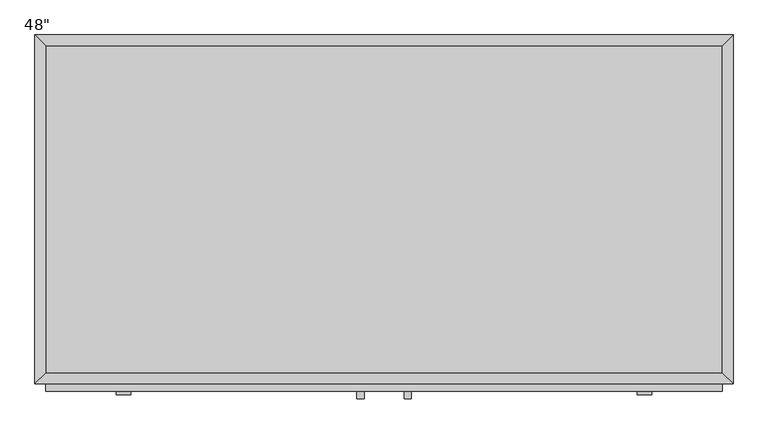
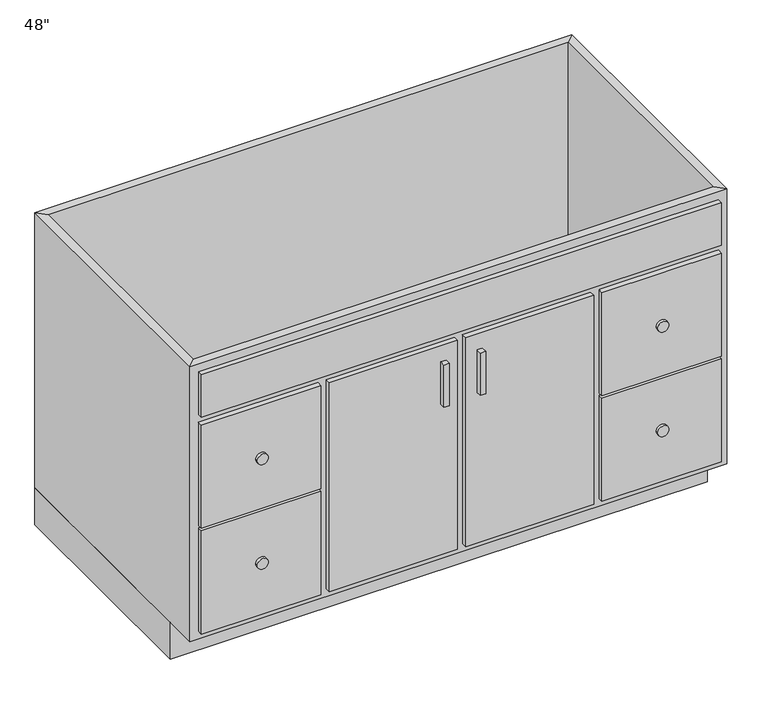
"""IFC4 building model written with IfcOpenShell, lengths in millimetres: furniture geometry."""

from ifc_helpers import new_model, si_unit, point, frame, frame_2d, origin, origin_with_axes, place, context, project, spatial, polyline, circle_curve, trimmed, segment, composite_curve, outline, extrude, faceted_brep, source, transform, mapped, element, save


def furniture_7e5e5cd5(model_context):
    return source(origin(), model_context, "Body", "SolidModel", [
        extrude(outline(polyline([(55.91996, -635.0), (43.21996, -635.0), (43.21996, -622.3), (55.91996, -622.3), (55.91996, -635.0)])), frame((0.0, 0.0, 469.9), z_axis=(0.0, 0.0, 1.0), x_axis=(1.0, 0.0, 0.0)), (0.0, 0.0, 1.0), 101.6),
        extrude(outline(polyline([(138.46996, -635.0), (125.76996, -635.0), (125.76996, -622.3), (138.46996, -622.3), (138.46996, -635.0)])), frame((0.0, 0.0, 469.9), z_axis=(0.0, 0.0, 1.0), x_axis=(1.0, 0.0, 0.0)), (0.0, 0.0, 1.0), 101.6),
        extrude(outline(composite_curve([segment(trimmed(circle_curve(frame_2d((484.1875, -363.97379)), 12.7), [point((484.1875, -376.67379))], [point((484.1875, -351.27379))], False, "CARTESIAN"), True, "CONTINUOUS"), segment(trimmed(circle_curve(frame_2d((484.1875, -363.97379)), 12.7), [point((484.1875, -351.27379))], [point((484.1875, -376.67379))], False, "CARTESIAN"), True, "CONTINUOUS")], self_intersect=False)), frame((0.0, -628.65, 0.0), z_axis=(0.0, 1.0, 0.0), x_axis=(0.0, 0.0, 1.0)), (0.0, 0.0, 1.0), 6.35),
        extrude(outline(composite_curve([segment(trimmed(circle_curve(frame_2d((233.3625, -363.97379)), 12.7), [point((233.3625, -376.67379))], [point((233.3625, -351.27379))], False, "CARTESIAN"), True, "CONTINUOUS"), segment(trimmed(circle_curve(frame_2d((233.3625, -363.97379)), 12.7), [point((233.3625, -351.27379))], [point((233.3625, -376.67379))], False, "CARTESIAN"), True, "CONTINUOUS")], self_intersect=False)), frame((0.0, -628.65, 0.0), z_axis=(0.0, 1.0, 0.0), x_axis=(0.0, 0.0, 1.0)), (0.0, 0.0, 1.0), 6.35),
        extrude(outline(composite_curve([segment(trimmed(circle_curve(frame_2d((233.3625, 545.66371)), 12.7), [point((233.3625, 532.96371))], [point((233.3625, 558.36371))], False, "CARTESIAN"), True, "CONTINUOUS"), segment(trimmed(circle_curve(frame_2d((233.3625, 545.66371)), 12.7), [point((233.3625, 558.36371))], [point((233.3625, 532.96371))], False, "CARTESIAN"), True, "CONTINUOUS")], self_intersect=False)), frame((0.0, -628.65, 0.0), z_axis=(0.0, 1.0, 0.0), x_axis=(0.0, 0.0, 1.0)), (0.0, 0.0, 1.0), 6.35),
        extrude(outline(composite_curve([segment(trimmed(circle_curve(frame_2d((484.1875, 545.66371)), 12.7), [point((484.1875, 532.96371))], [point((484.1875, 558.36371))], False, "CARTESIAN"), True, "CONTINUOUS"), segment(trimmed(circle_curve(frame_2d((484.1875, 545.66371)), 12.7), [point((484.1875, 558.36371))], [point((484.1875, 532.96371))], False, "CARTESIAN"), True, "CONTINUOUS")], self_intersect=False)), frame((0.0, -628.65, 0.0), z_axis=(0.0, 1.0, 0.0), x_axis=(0.0, 0.0, 1.0)), (0.0, 0.0, 1.0), 6.35),
        extrude(outline(polyline([(681.39496, -19.05), (681.39496, -590.55), (-499.70504, -590.55), (-499.70504, -19.05), (681.39496, -19.05)])), frame((0.0, 0.0, 88.9), z_axis=(0.0, 0.0, 1.0), x_axis=(1.0, 0.0, 0.0)), (0.0, 0.0, 1.0), 19.05),
        faceted_brep([(681.39496, -590.55, 749.3), (681.39496, -590.55, 88.9), (-499.70504, -590.55, 88.9), (-499.70504, -590.55, 749.3), (700.44496, -609.6, 749.3), (-518.75504, -609.6, 749.3), (700.44496, -609.6, 88.9), (-518.75504, -609.6, 88.9), (-499.70504, -19.05, 88.9), (-499.70504, -19.05, 749.3), (-518.75504, 0.0, 749.3), (-518.75504, 0.0, 88.9), (681.39496, -19.05, 88.9), (681.39496, -19.05, 749.3), (700.44496, 0.0, 749.3), (700.44496, 0.0, 88.9)], [[[0, 1, 2, 3]], [[4, 0, 3, 5]], [[6, 4, 5, 7]], [[1, 6, 7, 2]], [[3, 2, 8, 9]], [[5, 3, 9, 10]], [[7, 5, 10, 11]], [[2, 7, 11, 8]], [[9, 8, 12, 13]], [[10, 9, 13, 14]], [[11, 10, 14, 15]], [[8, 11, 15, 12]], [[13, 12, 1, 0]], [[14, 13, 0, 4]], [[15, 14, 4, 6]], [[12, 15, 6, 1]]]),
        extrude(outline(polyline([(700.44496, 0.0), (700.44496, -533.4), (-518.75504, -533.4), (-518.75504, 0.0), (700.44496, 0.0)])), origin_with_axes(), (0.0, 0.0, 1.0), 88.9),
        extrude(outline(polyline([(681.39496, -622.3), (-499.70504, -622.3), (-499.70504, -609.6), (681.39496, -609.6), (681.39496, -622.3)])), frame((0.0, 0.0, 628.65), z_axis=(0.0, 0.0, 1.0), x_axis=(1.0, 0.0, 0.0)), (0.0, 0.0, 1.0), 101.6),
        extrude(outline(polyline([(681.39496, -622.3), (409.93246, -622.3), (409.93246, -609.6), (681.39496, -609.6), (681.39496, -622.3)])), frame((0.0, 0.0, 361.95), z_axis=(0.0, 0.0, 1.0), x_axis=(1.0, 0.0, 0.0)), (0.0, 0.0, 1.0), 247.65),
        extrude(outline(polyline([(681.39496, -622.3), (409.93246, -622.3), (409.93246, -609.6), (681.39496, -609.6), (681.39496, -622.3)])), frame((0.0, 0.0, 107.95), z_axis=(0.0, 0.0, 1.0), x_axis=(1.0, 0.0, 0.0)), (0.0, 0.0, 1.0), 247.65),
        extrude(outline(polyline([(-228.24254, -622.3), (-499.70504, -622.3), (-499.70504, -609.6), (-228.24254, -609.6), (-228.24254, -622.3)])), frame((0.0, 0.0, 361.95), z_axis=(0.0, 0.0, 1.0), x_axis=(1.0, 0.0, 0.0)), (0.0, 0.0, 1.0), 247.65),
        extrude(outline(polyline([(-228.24254, -622.3), (-499.70504, -622.3), (-499.70504, -609.6), (-228.24254, -609.6), (-228.24254, -622.3)])), frame((0.0, 0.0, 107.95), z_axis=(0.0, 0.0, 1.0), x_axis=(1.0, 0.0, 0.0)), (0.0, 0.0, 1.0), 247.65),
        extrude(outline(polyline([(81.31996, -622.3), (-209.19254, -622.3), (-209.19254, -609.6), (81.31996, -609.6), (81.31996, -622.3)])), frame((0.0, 0.0, 107.95), z_axis=(0.0, 0.0, 1.0), x_axis=(1.0, 0.0, 0.0)), (0.0, 0.0, 1.0), 501.65),
        extrude(outline(polyline([(390.88246, -622.3), (100.36996, -622.3), (100.36996, -609.6), (390.88246, -609.6), (390.88246, -622.3)])), frame((0.0, 0.0, 107.95), z_axis=(0.0, 0.0, 1.0), x_axis=(1.0, 0.0, 0.0)), (0.0, 0.0, 1.0), 501.65),
    ])


if __name__ == "__main__":
    model = new_model("IFC4")
    model_context = context("Model", 3, world=origin())
    ifc_project = project(units=[si_unit("LENGTHUNIT", "METRE", prefix="MILLI")], contexts=[model_context])
    site = spatial("IfcSite", under=ifc_project)
    building = spatial("IfcBuilding", under=site)
    placement = place(None, origin())
    furniture_shape = furniture_7e5e5cd5(model_context)
    element("IfcFurniture", 1, ObjectType="48\"", at=placement, inside=building, context=model_context, shape_type="MappedRepresentation", body=[
        mapped(furniture_shape, transform((0.0, 0.0, 0.0), x_axis=(1.0, 0.0, 0.0), y_axis=(0.0, 1.0, 0.0), z_axis=(0.0, 0.0, 1.0))),
    ])
    save(model, "model.ifc")

# Revit data of these elements
# Type "48\""
#   Assembly Code = "C1030410"
#   Depth = 2' - 0"
#   Height = 2' - 5 1/2"
#   Toe Depth = 0' - 3"
#   Toe Height = 0' - 3 1/2"
#   Width = 4' - 0"
#   Cabinet Material = none
#   Door/Drawer Material = none
#   Handle Material = Cabinets - Handles
#   Default Elevation = 0
# Element 1 (IfcFurniture, "48\"")
#   Materials on its faces: "Cabinets", "Cabinets - Handles"
# Materials
#   "Cabinets - Handles": class "Metal", colour RGB 57 57 57, transparency 0
#   "Cabinets": colour RGB 249 249 249, transparency 0
